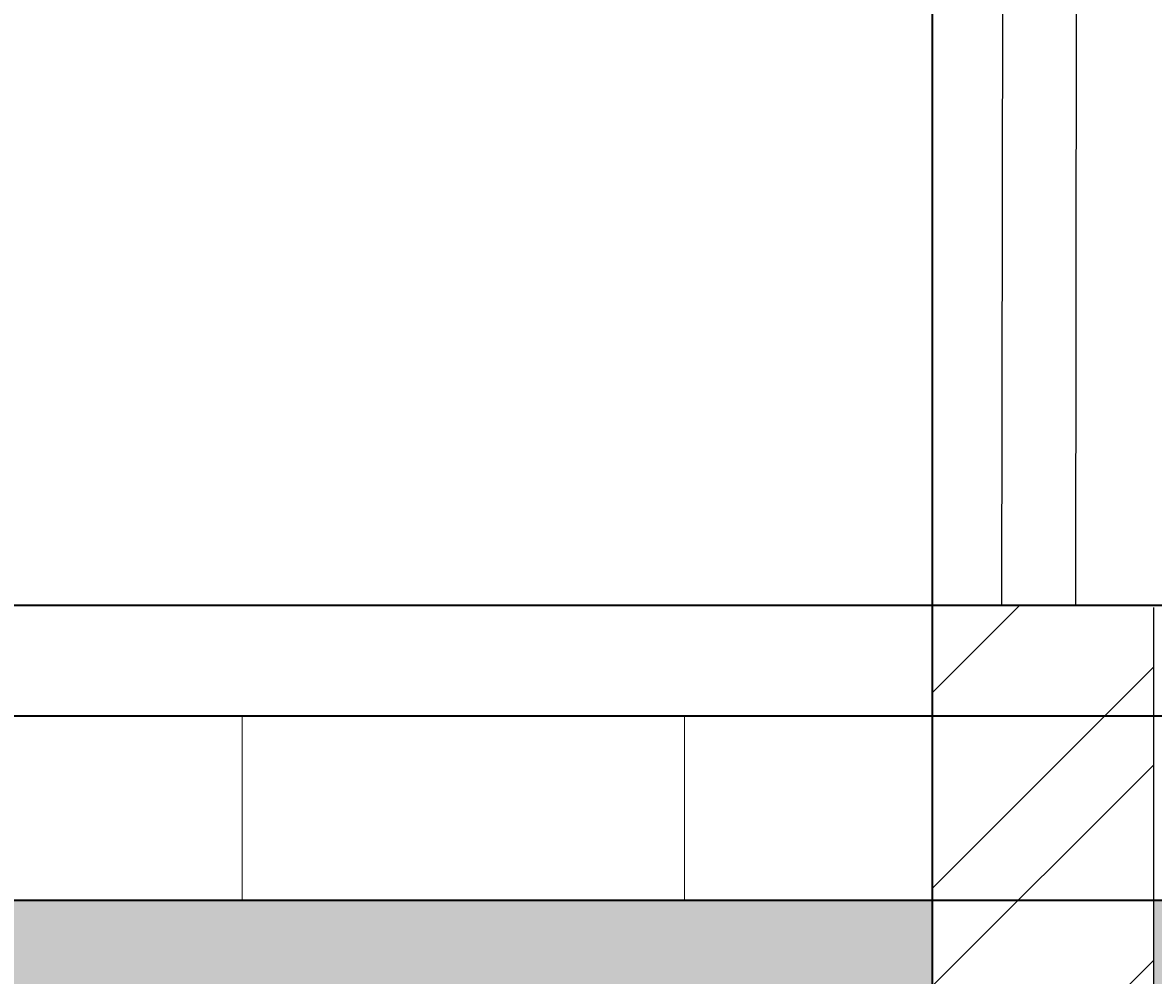
# Model space of a CAD drawing. Units: inches. Extents: x -301 to 715, y -607 to 364.
# Tile 18 of 141: x -66 to -35, y -474 to -448. Entities that reach past the tile are written whole.
import ezdxf

# ---------------------------------------------------------------- set-up
doc = ezdxf.new("R2010")
doc.units = ezdxf.units.IN
doc.header["$MEASUREMENT"] = 0
for name, color, linetype, lineweight in [('A-ANNO-DIMS', 2, 'Continuous', 18), ('A-DOOR', 4, 'Continuous', 25), ('A-SECT', 1, 'Continuous', 35), ('A-SECT-PATT', 8, 'Continuous', 13)]:
    doc.layers.add(name, color=color, linetype=linetype, lineweight=lineweight)
doc.styles.get("Standard").update_dxf_attribs({"font": 'arial.ttf'})
doc.dimstyles.get("Standard").update_dxf_attribs({"dimtxt": 0.18, "dimasz": 0.18, "dimexe": 0.18, "dimexo": 0.0625, "dimgap": 0.09, "dimtad": 0, "dimtih": 1, "dimtoh": 1, "dimdec": 1, "dimzin": 0, "dimdsep": 46, "dimlunit": 4, "dimtxsty": 'Standard', "dimcen": 0.09, "dimclrd": 3, "dimclre": 4, "dimclrt": 6, "dimadec": 0, "dimazin": 0, "dimtfac": 1, "dimtdec": 1, "dimtofl": 0, "dimtmove": 0, "dimatfit": 3, "dimfxl": 1, "dimtfill": 2, "dimtfillclr": 51, "dimtolj": 1, "dimtzin": 0, "dimarcsym": 0})

# ---------------------------------------------------------------- blocks, each defined once
blk = doc.blocks.new('*D179')
at = {"layer": 'A-ANNO-DIMS', "color": 4, "lineweight": -2, "transparency": 16777216}
for p, q in [((-87.981, -433.54), (-87.981, -573.809)), ((-35.282, -463.54), (-35.282, -573.809))]:
    blk.add_line(p, q, dxfattribs=at)
at = {"layer": 'A-ANNO-DIMS', "color": 3, "lineweight": -2, "transparency": 16777216}
for p, q in [((-87.801, -573.629), (-62.174, -573.629)), ((-35.462, -573.629), (-61.089, -573.629))]:
    blk.add_line(p, q, dxfattribs=at)
at = {"layer": 'A-ANNO-DIMS', "color": 3, "transparency": 16777216}
for points in [[(-87.801, -573.599), (-87.801, -573.659), (-87.981, -573.629)], [(-35.462, -573.599), (-35.462, -573.659), (-35.282, -573.629)]]:
    blk.add_solid(points, dxfattribs=at)
at = {"layer": 'Defpoints', "color": 0, "transparency": 16777216}
for p in [(-87.981, -433.477), (-35.282, -463.477), (-35.282, -573.629)]:
    blk.add_point(p, dxfattribs=at)
at = {"layer": 'A-ANNO-DIMS', "color": 6, "transparency": 16777216, "insert": (-61.631, -573.629), "char_height": 0.18, "attachment_point": 5, "bg_fill": 1, "box_fill_scale": 1.25, "bg_fill_color": 51, "bg_fill_transparency": 0}
blk.add_mtext('\\A1;4\'-4 1/2"', dxfattribs=at)
blk = doc.blocks.new('*D180')
at = {"layer": 'A-ANNO-DIMS', "color": 4, "lineweight": -2, "transparency": 16777216}
for p, q in [((-35.282, -463.54), (-35.282, -573.809)), ((12.718, -463.54), (12.718, -573.809))]:
    blk.add_line(p, q, dxfattribs=at)
at = {"layer": 'A-ANNO-DIMS', "color": 3, "lineweight": -2, "transparency": 16777216}
for p, q in [((-35.102, -573.629), (-11.615, -573.629)), ((12.538, -573.629), (-10.949, -573.629))]:
    blk.add_line(p, q, dxfattribs=at)
at = {"layer": 'A-ANNO-DIMS', "color": 3, "transparency": 16777216}
for points in [[(-35.102, -573.599), (-35.102, -573.659), (-35.282, -573.629)], [(12.538, -573.599), (12.538, -573.659), (12.718, -573.629)]]:
    blk.add_solid(points, dxfattribs=at)
at = {"layer": 'Defpoints', "color": 0, "transparency": 16777216}
for p in [(-35.282, -463.477), (12.718, -463.477), (12.718, -573.629)]:
    blk.add_point(p, dxfattribs=at)
at = {"layer": 'A-ANNO-DIMS', "color": 6, "transparency": 16777216, "insert": (-11.282, -573.629), "char_height": 0.18, "attachment_point": 5, "bg_fill": 1, "box_fill_scale": 1.25, "bg_fill_color": 51, "bg_fill_transparency": 0}
blk.add_mtext('\\A1;4\'-0"', dxfattribs=at)

msp = doc.modelspace()

# ---------------------------------------------------------------- hatches: boundary and pattern name
at = {"layer": 'A-SECT-PATT'}
h = msp.add_hatch(dxfattribs=at)
h.set_pattern_fill('ANSI32', color=256, scale=15)
h.set_pattern_definition([(45, (10.321, 33.8764), (-3.977476, 3.977476), []), (45, (12.973, 33.8764), (-3.977476, 3.977476), [])])
h.paths.add_polyline_path([(-185.282, -324.477), (-199.282, -324.477), (-199.282, -329.477), (-194.282, -329.477), (-194.282, -353.477), (-185.282, -353.477)])
h.paths.add_polyline_path([(-185.282, -361.477), (-193.904, -361.477), (-193.982, -377.537), (-185.282, -377.537)])
h.paths.add_polyline_path([(143.218, -329.477), (148.218, -329.477), (148.218, -324.477), (134.255, -324.477), (134.255, -353.477), (143.218, -353.477)])
h.paths.add_polyline_path([(143.218, -361.477), (134.255, -361.477), (134.255, -377.477), (143.218, -377.477)])
h.paths.add_polyline_path([(-185.282, -439.477), (-194.282, -439.477), (-194.282, -463.477), (-185.282, -463.477)])
h.paths.add_polyline_path([(-185.282, -471.477), (-194.282, -471.477), (-194.282, -481.477), (-185.282, -481.477)])
h.paths.add_polyline_path([(-185.282, -463.477), (-194.282, -463.477), (-194.282, -466.477), (-185.282, -466.477)])
h.paths.add_polyline_path([(-185.282, -466.477), (-194.282, -466.477), (-194.282, -471.477), (-185.282, -471.477)])
h.paths.add_polyline_path([(-180.282, -481.477), (-185.282, -481.477), (-194.282, -481.477), (-199.282, -481.477), (-199.282, -493.477), (-180.282, -493.477)])
h.paths.add_polyline_path([(-175.282, -493.477), (-180.282, -493.477), (-199.282, -493.477), (-204.282, -493.477), (-204.282, -511.477), (-175.282, -511.477)])
h.paths.add_polyline_path([(-170.282, -511.477), (-175.282, -511.477), (-204.282, -511.477), (-209.282, -511.477), (-209.282, -535.477), (-170.282, -535.477)])
h.paths.add_polyline_path([(-35.282, -463.477), (-41.282, -463.477), (-41.282, -466.477), (-35.282, -466.477)])
h.paths.add_polyline_path([(-35.282, -466.477), (-41.282, -466.477), (-41.282, -471.477), (-35.282, -471.477)])
h.paths.add_polyline_path([(-35.282, -471.477), (-41.282, -471.477), (-41.282, -481.477), (-35.282, -481.477)])
h.paths.add_polyline_path([(-30.282, -481.477), (-46.282, -481.477), (-46.282, -493.477), (-30.282, -493.477)])
h.paths.add_polyline_path([(-25.282, -493.477), (-30.282, -493.477), (-46.282, -493.477), (-51.282, -493.477), (-51.282, -511.477), (-25.282, -511.477)])
h.paths.add_polyline_path([(-20.282, -511.477), (-25.282, -511.477), (-51.282, -511.477), (-56.282, -511.477), (-56.282, -535.477), (-20.282, -535.477)])
h.paths.add_polyline_path([(143.218, -463.477), (134.255, -463.477), (134.255, -466.477), (143.218, -466.477)])
h.paths.add_polyline_path([(143.218, -466.477), (134.255, -466.477), (134.255, -471.477), (143.218, -471.477)])
h.paths.add_polyline_path([(143.218, -471.477), (134.255, -471.477), (134.255, -481.477), (143.218, -481.477)])
h.paths.add_polyline_path([(148.255, -481.477), (143.255, -481.477), (134.255, -481.477), (129.255, -481.477), (129.255, -493.477), (148.255, -493.477)])
h.paths.add_polyline_path([(153.255, -493.477), (148.255, -493.477), (129.255, -493.477), (124.255, -493.477), (124.255, -511.477), (153.255, -511.477)])
h.paths.add_polyline_path([(158.255, -511.477), (153.255, -511.477), (124.255, -511.477), (119.255, -511.477), (119.255, -535.477), (158.255, -535.477)])
h = msp.add_hatch(dxfattribs=at)
h.set_pattern_fill('AR-CONC', color=256, scale=0.5)
h.set_pattern_definition([(50, (10.3213, 33.8764), (3.586301, -0.31376), [0.375, -4.125]), (355, (10.3213, 33.8764), (-0.693757, 3.76096), [0.3, -3.3]), (100.45144, (10.62, 33.8502), (2.892544, 3.4472), [0.3187, -3.50571]), (46.1842, (10.3213, 34.8764), (5.336207, -0.827596), [0.5625, -6.1875]), (96.6356, (10.766, 34.8074), (4.67331, 4.870593), [0.47805, -5.25857]), (351.1842, (10.321, 34.8764), (4.67331, 4.870593), [0.45, -4.95]), (21, (10.8213, 34.6264), (2.984535, -2.013094), [0.375, -4.125]), (326, (10.8213, 34.6264), (1.216577, 3.62575), [0.3, -3.3]), (71.45144, (11.07, 34.4586), (4.201112, 1.612656), [0.3187, -3.50571]), (37.5, (10.3213, 33.8764), (0.0607993, 1.6644693), [0, -3.26, 0, -3.35, 0, -3.3125]), (7.5, (10.3213, 33.8764), (1.3153477, 1.9720586), [0, -1.91, 0, -3.185, 0, -1.2625]), (327.5, (9.2063, 33.8764), (2.6691122, -0.1127744), [0, -1.25, 0, -3.9, 0, -5.175]), (317.5, (8.7063, 33.8764), (2.915931, 0.500525), [0, -1.625, 0, -2.59, 0, -3.675])])
h.paths.add_polyline_path([(-56.282, -535.477), (-61.282, -535.477), (-61.282, -540.477), (-15.282, -540.477), (-15.282, -535.477), (-20.282, -535.477)])
h.paths.add_polyline_path([(119.255, -535.477), (114.255, -535.477), (114.255, -540.477), (163.255, -540.477), (163.255, -535.477), (158.255, -535.477)])
h.paths.add_polyline_path([(-206.282, -471.477), (-209.282, -471.477), (-209.282, -481.477), (-206.282, -481.477), (-194.282, -481.477), (-194.282, -471.477)])
h.paths.add_polyline_path([(-41.282, -481.477), (-41.282, -471.477), (-185.282, -471.477), (-185.282, -481.477), (-180.282, -481.477)])
h.paths.add_polyline_path([(134.255, -481.477), (134.255, -471.477), (-35.282, -471.477), (-35.282, -481.477), (-30.282, -481.477)])
h.paths.add_polyline_path([(155.218, -481.477), (158.218, -481.477), (158.218, -471.477), (153.218, -471.477), (143.218, -471.477), (143.218, -481.477), (148.255, -481.477)])
h.paths.add_polyline_path([(-193.88, -356.477), (-193.904, -361.477), (143.218, -361.477), (143.218, -356.477)])
h = msp.add_hatch(dxfattribs=at)
h.set_pattern_fill('ANSI31', color=256, scale=96, angle=45, style=0)
h.paths.add_polyline_path([(-185.282, -471.477), (-41.282, -471.477), (-41.282, -466.477), (-185.282, -466.477)])

# ---------------------------------------------------------------- linework, layer by layer
at = {"layer": 'A-DOOR'}
for p, q in [((-39.282, -385.476), (-39.396, -463.476)), ((-37.282, -385.479), (-37.396, -463.479))]:
    msp.add_line(p, q, dxfattribs=at)
at = {"layer": 'A-SECT'}
for p, q in [((-41.282, -361.477), (-41.282, -481.477)), ((-199.282, -463.477), (148.255, -463.477)), ((-204.282, -466.477), (153.218, -466.477)), ((-41.282, -466.477), (-41.282, -471.477)), ((-206.282, -471.477), (155.218, -471.477))]:
    msp.add_line(p, q, dxfattribs=at)

# ---------------------------------------------------------------- dimensions: what is measured, and where the dimension line sits
at = {"layer": 'A-ANNO-DIMS'}
for base, p1, p2, picture, middle in [((-35.282, -573.629), (-87.981, -433.477), (-35.282, -463.477), '*D179', (-61.631, -573.629)), ((12.718, -573.629), (-35.282, -463.477), (12.718, -463.477), '*D180', (-11.282, -573.629))]:
    dim = msp.add_linear_dim(base=base, p1=p1, p2=p2, dimstyle='Standard', override={"dimdec": 1, "dimlfac": 1, "dimrnd": 0, "dimzin": 1, "dimdsep": 46, "dimlunit": 4, "dimfrac": 2}, dxfattribs=at)
    dim.commit()
    dim.dimension.update_dxf_attribs({"geometry": picture, "text_midpoint": middle})

doc.saveas('drawing.dxf')
